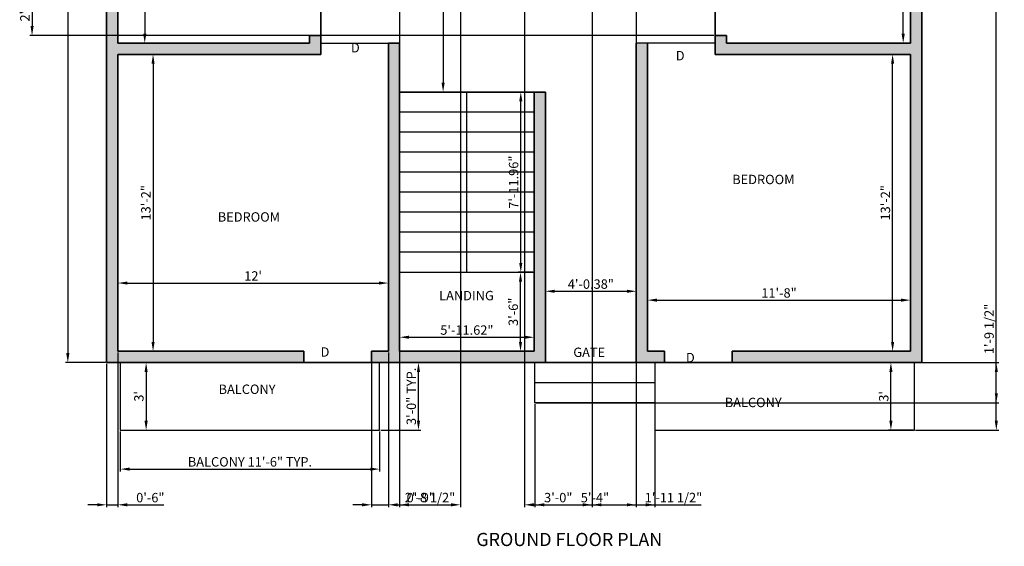
# Model space of a CAD drawing. Units: inches. Extents: x -48 to 476, y -487 to 101.
# Tile 1 of 2: x -48 to 476, y -487 to -207. Entities that reach past the tile are written whole.
import ezdxf

# ---------------------------------------------------------------- set-up
doc = ezdxf.new("R2010")
doc.units = ezdxf.units.IN
for name, color, linetype, lineweight in [('A-ANNO-DIMS', 2, 'Continuous', 18), ('A-ANNO-TEXT', 7, 'Continuous', 18), ('A-AREA-IDEN', 7, 'Continuous', 18), ('A-DOOR', 4, 'Continuous', 25), ('A-FLOR-BALC', 7, 'Continuous', 25), ('A-FLOR-STRS', 7, 'Continuous', 25), ('A-WALL', 7, 'Continuous', 35), ('A-WALL-PATT', 1, 'Continuous', 13)]:
    doc.layers.add(name, color=color, linetype=linetype, lineweight=lineweight)
doc.styles.get("Standard").update_dxf_attribs({"font": 'arial.ttf'})
doc.dimstyles.new('ISO-25', dxfattribs={"dimtxt": 5, "dimasz": 5, "dimexe": 1.25, "dimexo": 0.625, "dimtad": 1, "dimlunit": 3, "dimtxsty": 'Standard', "dimcen": 2.5, "dimadec": 0, "dimazin": 0, "dimtfac": 1, "dimtmove": 0, "dimatfit": 3, "dimfxl": 1, "dimarcsym": 0})

# ---------------------------------------------------------------- blocks, each defined once
blk = doc.blocks.new('*D9')
at = {"layer": 'A-ANNO-DIMS', "color": 0, "lineweight": -2, "transparency": 16777216}
for p, q in [((425.39, -159.13), (420.87, -159.13)), ((422.12, -214.13), (422.12, -164.13)), ((425.39, -219.13), (420.87, -219.13))]:
    blk.add_line(p, q, dxfattribs=at)
at = {"layer": 'A-ANNO-DIMS', "color": 0, "transparency": 16777216}
for points in [[(421.29, -164.13), (422.95, -164.13), (422.12, -159.13)], [(421.29, -214.13), (422.95, -214.13), (422.12, -219.13)]]:
    blk.add_solid(points, dxfattribs=at)
at = {"layer": 'Defpoints', "color": 0, "transparency": 16777216}
for p in [(422.12, -159.13), (426.01, -159.13), (426.01, -219.13)]:
    blk.add_point(p, dxfattribs=at)
at = {"layer": 'A-ANNO-DIMS', "color": 0, "transparency": 16777216, "insert": (418.95, -189.13), "char_height": 5, "attachment_point": 5, "rotation": 90}
blk.add_mtext("5'", dxfattribs=at)
blk = doc.blocks.new('*D10')
at = {"layer": 'A-ANNO-DIMS', "color": 0, "lineweight": -2, "transparency": 16777216}
for p, q in [((286.01, -382.51), (286.01, -354.68)), ((291.01, -355.93), (421.01, -355.93)), ((426.01, -382.51), (426.01, -354.68))]:
    blk.add_line(p, q, dxfattribs=at)
at = {"layer": 'A-ANNO-DIMS', "color": 0, "transparency": 16777216}
for points in [[(291.01, -355.1), (291.01, -356.77), (286.01, -355.93)], [(421.01, -355.1), (421.01, -356.77), (426.01, -355.93)]]:
    blk.add_solid(points, dxfattribs=at)
at = {"layer": 'Defpoints', "color": 0, "transparency": 16777216}
for p in [(426.01, -355.93), (286.01, -383.13), (426.01, -383.13)]:
    blk.add_point(p, dxfattribs=at)
at = {"layer": 'A-ANNO-DIMS', "color": 0, "transparency": 16777216, "insert": (356.01, -352.75), "char_height": 5, "attachment_point": 5}
blk.add_mtext('11\'-8"', dxfattribs=at)
blk = doc.blocks.new('*D11')
at = {"layer": 'A-ANNO-DIMS', "color": 0, "lineweight": -2, "transparency": 16777216}
for p, q in [((425.39, -225.13), (415.24, -225.13)), ((416.49, -378.13), (416.49, -230.13)), ((425.39, -383.13), (415.24, -383.13))]:
    blk.add_line(p, q, dxfattribs=at)
at = {"layer": 'A-ANNO-DIMS', "color": 0, "transparency": 16777216}
for points in [[(415.66, -230.13), (417.32, -230.13), (416.49, -225.13)], [(415.66, -378.13), (417.32, -378.13), (416.49, -383.13)]]:
    blk.add_solid(points, dxfattribs=at)
at = {"layer": 'Defpoints', "color": 0, "transparency": 16777216}
for p in [(416.49, -225.13), (426.01, -225.13), (426.01, -383.13)]:
    blk.add_point(p, dxfattribs=at)
at = {"layer": 'A-ANNO-DIMS', "color": 0, "transparency": 16777216, "insert": (413.31, -304.13), "char_height": 5, "attachment_point": 5, "rotation": 90}
blk.add_mtext('13\'-2"', dxfattribs=at)
blk = doc.blocks.new('*D12')
at = {"layer": 'A-ANNO-DIMS', "color": 0, "lineweight": -2, "transparency": 16777216}
for p, q in [((431.39, -389.13), (414.33, -389.13)), ((415.58, -420.13), (415.58, -394.13)), ((427.51, -425.13), (414.33, -425.13))]:
    blk.add_line(p, q, dxfattribs=at)
at = {"layer": 'A-ANNO-DIMS', "color": 0, "transparency": 16777216}
for points in [[(414.75, -394.13), (416.42, -394.13), (415.58, -389.13)], [(414.75, -420.13), (416.42, -420.13), (415.58, -425.13)]]:
    blk.add_solid(points, dxfattribs=at)
at = {"layer": 'Defpoints', "color": 0, "transparency": 16777216}
for p in [(415.58, -389.13), (432.01, -389.13), (428.14, -425.13)]:
    blk.add_point(p, dxfattribs=at)
at = {"layer": 'A-ANNO-DIMS', "color": 0, "transparency": 16777216, "insert": (412.4, -407.13), "char_height": 5, "attachment_point": 5, "rotation": 90}
blk.add_mtext("3'", dxfattribs=at)
blk = doc.blocks.new('*D13')
at = {"layer": 'A-ANNO-DIMS', "color": 0, "lineweight": -2, "transparency": 16777216}
for p, q in [((231.63, -350.58), (231.63, -349.96)), ((236.63, -351.21), (275.01, -351.21)), ((280.01, -350.58), (280.01, -349.96))]:
    blk.add_line(p, q, dxfattribs=at)
at = {"layer": 'A-ANNO-DIMS', "color": 0, "transparency": 16777216}
for points in [[(236.63, -350.37), (236.63, -352.04), (231.63, -351.21)], [(275.01, -350.37), (275.01, -352.04), (280.01, -351.21)]]:
    blk.add_solid(points, dxfattribs=at)
at = {"layer": 'Defpoints', "color": 0, "transparency": 16777216}
for p in [(231.63, -351.21), (280.01, -351.21), (280.01, -351.21)]:
    blk.add_point(p, dxfattribs=at)
at = {"layer": 'A-ANNO-DIMS', "color": 0, "transparency": 16777216, "insert": (255.82, -348.03), "char_height": 5, "attachment_point": 5}
blk.add_mtext('4\'-0.38"', dxfattribs=at)
blk = doc.blocks.new('*D14')
at = {"layer": 'A-ANNO-DIMS', "color": 0, "lineweight": -2, "transparency": 16777216}
for p, q in [((154.01, -382.51), (154.01, -374.42)), ((159.01, -375.67), (220.63, -375.67)), ((225.63, -382.51), (225.63, -374.42))]:
    blk.add_line(p, q, dxfattribs=at)
at = {"layer": 'A-ANNO-DIMS', "color": 0, "transparency": 16777216}
for points in [[(159.01, -374.84), (159.01, -376.5), (154.01, -375.67)], [(220.63, -374.84), (220.63, -376.5), (225.63, -375.67)]]:
    blk.add_solid(points, dxfattribs=at)
at = {"layer": 'Defpoints', "color": 0, "transparency": 16777216}
for p in [(225.63, -375.67), (154.01, -383.13), (225.63, -383.13)]:
    blk.add_point(p, dxfattribs=at)
at = {"layer": 'A-ANNO-DIMS', "color": 0, "transparency": 16777216, "insert": (189.82, -372.49), "char_height": 5, "attachment_point": 5}
blk.add_mtext('5\'-11.62"', dxfattribs=at)
blk = doc.blocks.new('*D15')
at = {"layer": 'A-ANNO-DIMS', "color": 0, "lineweight": -2, "transparency": 16777216}
for p, q in [((225.01, -341.13), (217.11, -341.13)), ((218.36, -378.13), (218.36, -346.13)), ((225.01, -383.13), (217.11, -383.13))]:
    blk.add_line(p, q, dxfattribs=at)
at = {"layer": 'A-ANNO-DIMS', "color": 0, "transparency": 16777216}
for points in [[(217.53, -346.13), (219.2, -346.13), (218.36, -341.13)], [(217.53, -378.13), (219.2, -378.13), (218.36, -383.13)]]:
    blk.add_solid(points, dxfattribs=at)
at = {"layer": 'Defpoints', "color": 0, "transparency": 16777216}
for p in [(218.36, -341.13), (225.63, -341.13), (225.63, -383.13)]:
    blk.add_point(p, dxfattribs=at)
at = {"layer": 'A-ANNO-DIMS', "color": 0, "transparency": 16777216, "insert": (215.18, -362.13), "char_height": 5, "attachment_point": 5, "rotation": 90}
blk.add_mtext('3\'-6"', dxfattribs=at)
blk = doc.blocks.new('*D16')
at = {"layer": 'A-ANNO-DIMS', "color": 0, "lineweight": -2, "transparency": 16777216}
for p, q in [((225.01, -245.18), (217.26, -245.18)), ((218.51, -336.13), (218.51, -250.18)), ((225.01, -341.13), (217.26, -341.13))]:
    blk.add_line(p, q, dxfattribs=at)
at = {"layer": 'A-ANNO-DIMS', "color": 0, "transparency": 16777216}
for points in [[(217.68, -250.18), (219.34, -250.18), (218.51, -245.18)], [(217.68, -336.13), (219.34, -336.13), (218.51, -341.13)]]:
    blk.add_solid(points, dxfattribs=at)
at = {"layer": 'Defpoints', "color": 0, "transparency": 16777216}
for p in [(218.51, -245.18), (225.63, -245.18), (225.63, -341.13)]:
    blk.add_point(p, dxfattribs=at)
at = {"layer": 'A-ANNO-DIMS', "color": 0, "transparency": 16777216, "insert": (215.33, -293.15), "char_height": 5, "attachment_point": 5, "rotation": 90}
blk.add_mtext('7\'-11.96"', dxfattribs=at)
blk = doc.blocks.new('*D17')
at = {"layer": 'A-ANNO-DIMS', "color": 0, "lineweight": -2, "transparency": 16777216}
for p, q in [((5.92, -389.13), (20.28, -389.13)), ((19.03, -394.13), (19.03, -420.13)), ((5.92, -425.13), (20.28, -425.13))]:
    blk.add_line(p, q, dxfattribs=at)
at = {"layer": 'A-ANNO-DIMS', "color": 0, "transparency": 16777216}
for points in [[(18.2, -394.13), (19.87, -394.13), (19.03, -389.13)], [(18.2, -420.13), (19.87, -420.13), (19.03, -425.13)]]:
    blk.add_solid(points, dxfattribs=at)
at = {"layer": 'Defpoints', "color": 0, "transparency": 16777216}
for p in [(5.3, -389.13), (5.3, -425.13), (19.03, -425.13)]:
    blk.add_point(p, dxfattribs=at)
at = {"layer": 'A-ANNO-DIMS', "color": 0, "transparency": 16777216, "insert": (15.85, -407.13), "char_height": 5, "attachment_point": 5, "rotation": 90}
blk.add_mtext("3'", dxfattribs=at)
blk = doc.blocks.new('*D18')
at = {"layer": 'A-ANNO-DIMS', "color": 0, "lineweight": -2, "transparency": 16777216}
for p, q in [((4.01, -382.51), (4.01, -345.58)), ((148.01, -382.51), (148.01, -345.58)), ((9.01, -346.83), (143.01, -346.83))]:
    blk.add_line(p, q, dxfattribs=at)
at = {"layer": 'A-ANNO-DIMS', "color": 0, "transparency": 16777216}
for points in [[(9.01, -346), (9.01, -347.67), (4.01, -346.83)], [(143.01, -346), (143.01, -347.67), (148.01, -346.83)]]:
    blk.add_solid(points, dxfattribs=at)
at = {"layer": 'Defpoints', "color": 0, "transparency": 16777216}
for p in [(148.01, -346.83), (4.01, -383.13), (148.01, -383.13)]:
    blk.add_point(p, dxfattribs=at)
at = {"layer": 'A-ANNO-DIMS', "color": 0, "transparency": 16777216, "insert": (76.01, -343.7), "char_height": 5, "attachment_point": 5}
blk.add_mtext("12'", dxfattribs=at)
blk = doc.blocks.new('*D19')
at = {"layer": 'A-ANNO-DIMS', "color": 0, "lineweight": -2, "transparency": 16777216}
for p, q in [((4.64, -225.13), (23.98, -225.13)), ((22.73, -230.13), (22.73, -378.13)), ((4.64, -383.13), (23.98, -383.13))]:
    blk.add_line(p, q, dxfattribs=at)
at = {"layer": 'A-ANNO-DIMS', "color": 0, "transparency": 16777216}
for points in [[(21.9, -230.13), (23.56, -230.13), (22.73, -225.13)], [(21.9, -378.13), (23.56, -378.13), (22.73, -383.13)]]:
    blk.add_solid(points, dxfattribs=at)
at = {"layer": 'Defpoints', "color": 0, "transparency": 16777216}
for p in [(4.01, -225.13), (4.01, -383.13), (22.73, -383.13)]:
    blk.add_point(p, dxfattribs=at)
at = {"layer": 'A-ANNO-DIMS', "color": 0, "transparency": 16777216, "insert": (19.55, -304.13), "char_height": 5, "attachment_point": 5, "rotation": 90}
blk.add_mtext('13\'-2"', dxfattribs=at)
blk = doc.blocks.new('*D21')
at = {"layer": 'A-ANNO-DIMS', "color": 0, "lineweight": -2, "transparency": 16777216}
for p, q in [((4.64, -159.13), (19.56, -159.13)), ((18.31, -164.13), (18.31, -214.13)), ((4.64, -219.13), (19.56, -219.13))]:
    blk.add_line(p, q, dxfattribs=at)
at = {"layer": 'A-ANNO-DIMS', "color": 0, "transparency": 16777216}
for points in [[(17.48, -164.13), (19.15, -164.13), (18.31, -159.13)], [(17.48, -214.13), (19.15, -214.13), (18.31, -219.13)]]:
    blk.add_solid(points, dxfattribs=at)
at = {"layer": 'Defpoints', "color": 0, "transparency": 16777216}
for p in [(4.01, -159.13), (4.01, -219.13), (18.31, -219.13)]:
    blk.add_point(p, dxfattribs=at)
at = {"layer": 'A-ANNO-DIMS', "color": 0, "transparency": 16777216, "insert": (15.14, -189.13), "char_height": 5, "attachment_point": 5, "rotation": 90}
blk.add_mtext("5'", dxfattribs=at)
blk = doc.blocks.new('*D22')
at = {"layer": 'A-ANNO-DIMS', "color": 0, "lineweight": -2, "transparency": 16777216}
for p, q in [((154.64, -93.13), (178.42, -93.13)), ((177.17, -98.13), (177.17, -240.18)), ((154.64, -245.18), (178.42, -245.18))]:
    blk.add_line(p, q, dxfattribs=at)
at = {"layer": 'A-ANNO-DIMS', "color": 0, "transparency": 16777216}
for points in [[(176.34, -98.13), (178, -98.13), (177.17, -93.13)], [(176.34, -240.18), (178, -240.18), (177.17, -245.18)]]:
    blk.add_solid(points, dxfattribs=at)
at = {"layer": 'Defpoints', "color": 0, "transparency": 16777216}
for p in [(154.01, -93.13), (154.01, -245.18), (177.17, -245.18)]:
    blk.add_point(p, dxfattribs=at)
at = {"layer": 'A-ANNO-DIMS', "color": 0, "transparency": 16777216, "insert": (173.99, -169.15), "char_height": 5, "attachment_point": 5, "rotation": 90}
blk.add_mtext('12\'-8.04"', dxfattribs=at)
blk = doc.blocks.new('*D26')
at = {"layer": 'A-ANNO-DIMS', "color": 0, "lineweight": -2, "transparency": 16777216}
for p, q in [((-2.61, 14.87), (-23.89, 14.87)), ((-22.64, 9.87), (-22.64, -384.13)), ((-2.61, -389.13), (-23.89, -389.13))]:
    blk.add_line(p, q, dxfattribs=at)
at = {"layer": 'A-ANNO-DIMS', "color": 0, "transparency": 16777216}
for points in [[(-23.48, 9.87), (-21.81, 9.87), (-22.64, 14.87)], [(-23.48, -384.13), (-21.81, -384.13), (-22.64, -389.13)]]:
    blk.add_solid(points, dxfattribs=at)
at = {"layer": 'Defpoints', "color": 0, "transparency": 16777216}
for p in [(-1.99, 14.87), (-22.64, -389.13), (-1.99, -389.13)]:
    blk.add_point(p, dxfattribs=at)
at = {"layer": 'A-ANNO-DIMS', "color": 0, "transparency": 16777216, "insert": (-25.82, -187.13), "char_height": 5, "attachment_point": 5, "rotation": 90}
blk.add_mtext('33\'-8"', dxfattribs=at)
blk = doc.blocks.new('BALCONY-EDGE-REAR')
for p, q in [((0, 0), (0, -36)), ((138.05, -36), (138.05, 0)), ((0, -36), (138.05, -36))]:
    blk.add_line(p, q)
blk = doc.blocks.new('DOOR-36-CLOSED')
blk.add_line((0, 0), (36, 0))
blk = doc.blocks.new('*D31')
at = {"layer": 'A-ANNO-DIMS', "color": 0, "lineweight": -2, "transparency": 16777216}
for p, q in [((5.3, -425.76), (5.3, -447.09)), ((143.34, -425.76), (143.34, -447.09)), ((10.3, -445.84), (138.34, -445.84))]:
    blk.add_line(p, q, dxfattribs=at)
at = {"layer": 'A-ANNO-DIMS', "color": 0, "transparency": 16777216}
for points in [[(10.3, -445.01), (10.3, -446.67), (5.3, -445.84)], [(138.34, -445.01), (138.34, -446.67), (143.34, -445.84)]]:
    blk.add_solid(points, dxfattribs=at)
at = {"layer": 'Defpoints', "color": 0, "transparency": 16777216}
for p in [(5.3, -425.13), (143.34, -425.13), (143.34, -445.84)]:
    blk.add_point(p, dxfattribs=at)
at = {"layer": 'A-ANNO-DIMS', "color": 0, "transparency": 16777216, "insert": (74.32, -442.63), "char_height": 5, "attachment_point": 5}
blk.add_mtext('BALCONY 11\'-6" TYP.', dxfattribs=at)
blk = doc.blocks.new('*D32')
at = {"layer": 'A-ANNO-DIMS', "color": 0, "lineweight": -2, "transparency": 16777216}
for p, q in [((143.97, -389.13), (165.3, -389.13)), ((164.05, -420.13), (164.05, -394.13)), ((143.97, -425.13), (165.3, -425.13))]:
    blk.add_line(p, q, dxfattribs=at)
at = {"layer": 'A-ANNO-DIMS', "color": 0, "transparency": 16777216}
for points in [[(163.22, -394.13), (164.88, -394.13), (164.05, -389.13)], [(163.22, -420.13), (164.88, -420.13), (164.05, -425.13)]]:
    blk.add_solid(points, dxfattribs=at)
at = {"layer": 'Defpoints', "color": 0, "transparency": 16777216}
for p in [(143.34, -389.13), (164.05, -389.13), (143.34, -425.13)]:
    blk.add_point(p, dxfattribs=at)
at = {"layer": 'A-ANNO-DIMS', "color": 0, "transparency": 16777216, "insert": (160.87, -407.13), "char_height": 5, "attachment_point": 5, "rotation": 90}
blk.add_mtext('3\'-0" TYP.', dxfattribs=at)
blk = doc.blocks.new('*D33')
at = {"layer": 'A-ANNO-DIMS', "color": 0, "lineweight": -2, "transparency": 16777216}
for p, q in [((428.77, 50.87), (472.96, 50.87)), ((471.71, -420.13), (471.71, 45.87)), ((428.76, -425.13), (472.96, -425.13))]:
    blk.add_line(p, q, dxfattribs=at)
at = {"layer": 'A-ANNO-DIMS', "color": 0, "transparency": 16777216}
for points in [[(470.88, 45.87), (472.54, 45.87), (471.71, 50.87)], [(470.88, -420.13), (472.54, -420.13), (471.71, -425.13)]]:
    blk.add_solid(points, dxfattribs=at)
at = {"layer": 'Defpoints', "color": 0, "transparency": 16777216}
for p in [(428.14, 50.87), (471.71, 50.87), (428.14, -425.13)]:
    blk.add_point(p, dxfattribs=at)
at = {"layer": 'A-ANNO-DIMS', "color": 0, "transparency": 16777216, "insert": (468.53, -187.13), "char_height": 5, "attachment_point": 5, "rotation": 90}
blk.add_mtext('39\'-8"', dxfattribs=at)
blk = doc.blocks.new('*D36')
at = {"layer": 'A-ANNO-DIMS', "color": 0, "lineweight": -2, "transparency": 16777216}
for p, q in [((154.01, -87.76), (154.01, -466.08)), ((186.37, -87.76), (186.37, -466.08)), ((159.01, -464.83), (181.37, -464.83))]:
    blk.add_line(p, q, dxfattribs=at)
at = {"layer": 'A-ANNO-DIMS', "color": 0, "transparency": 16777216}
for points in [[(159.01, -464), (159.01, -465.67), (154.01, -464.83)], [(181.37, -464), (181.37, -465.67), (186.37, -464.83)]]:
    blk.add_solid(points, dxfattribs=at)
at = {"layer": 'Defpoints', "color": 0, "transparency": 16777216}
for p in [(154.01, -87.13), (186.37, -87.13), (186.37, -464.83)]:
    blk.add_point(p, dxfattribs=at)
at = {"layer": 'A-ANNO-DIMS', "color": 0, "transparency": 16777216, "insert": (170.19, -461.62), "char_height": 5, "attachment_point": 5}
blk.add_mtext('2\'-8 1/2"', dxfattribs=at)
blk = doc.blocks.new('*D37')
at = {"layer": 'A-ANNO-DIMS', "color": 0, "lineweight": -2, "transparency": 16777216}
for p, q in [((256.47, -87.76), (256.47, -466.08)), ((280.01, -87.76), (280.01, -466.08)), ((261.47, -464.83), (275.01, -464.83)), ((280.01, -464.83), (314.62, -464.83))]:
    blk.add_line(p, q, dxfattribs=at)
at = {"layer": 'A-ANNO-DIMS', "color": 0, "transparency": 16777216}
for points in [[(261.47, -464), (261.47, -465.67), (256.47, -464.83)], [(275.01, -464), (275.01, -465.67), (280.01, -464.83)]]:
    blk.add_solid(points, dxfattribs=at)
at = {"layer": 'Defpoints', "color": 0, "transparency": 16777216}
for p in [(256.47, -87.13), (280.01, -87.13), (280.01, -464.83)]:
    blk.add_point(p, dxfattribs=at)
at = {"layer": 'A-ANNO-DIMS', "color": 0, "transparency": 16777216, "insert": (299.81, -461.62), "char_height": 5, "attachment_point": 5}
blk.add_mtext('1\'-11 1/2"', dxfattribs=at)
blk = doc.blocks.new('*D39')
at = {"layer": 'A-ANNO-DIMS', "color": 0, "lineweight": -2, "transparency": 16777216}
for p, q in [((220.47, -93.76), (220.47, -466.08)), ((256.47, -93.76), (256.47, -466.08)), ((225.47, -464.83), (251.47, -464.83))]:
    blk.add_line(p, q, dxfattribs=at)
at = {"layer": 'A-ANNO-DIMS', "color": 0, "transparency": 16777216}
for points in [[(225.47, -464), (225.47, -465.67), (220.47, -464.83)], [(251.47, -464), (251.47, -465.67), (256.47, -464.83)]]:
    blk.add_solid(points, dxfattribs=at)
at = {"layer": 'Defpoints', "color": 0, "transparency": 16777216}
for p in [(220.47, -93.13), (256.47, -93.13), (256.47, -464.83)]:
    blk.add_point(p, dxfattribs=at)
at = {"layer": 'A-ANNO-DIMS', "color": 0, "transparency": 16777216, "insert": (238.47, -461.65), "char_height": 5, "attachment_point": 5}
blk.add_mtext('3\'-0"', dxfattribs=at)
blk = doc.blocks.new('*D40')
at = {"layer": 'A-ANNO-DIMS', "color": 0, "lineweight": -2, "transparency": 16777216}
for p, q in [((4.01, -383.76), (4.01, -466.08)), ((-1.99, -389.76), (-1.99, -466.08)), ((-6.99, -464.83), (-11.99, -464.83)), ((-1.99, -464.83), (4.01, -464.83)), ((9.01, -464.83), (28.55, -464.83))]:
    blk.add_line(p, q, dxfattribs=at)
at = {"layer": 'A-ANNO-DIMS', "color": 0, "transparency": 16777216}
for points in [[(-6.99, -464), (-6.99, -465.67), (-1.99, -464.83)], [(9.01, -464), (9.01, -465.67), (4.01, -464.83)]]:
    blk.add_solid(points, dxfattribs=at)
at = {"layer": 'Defpoints', "color": 0, "transparency": 16777216}
for p in [(4.01, -383.13), (-1.99, -389.13), (4.01, -464.83)]:
    blk.add_point(p, dxfattribs=at)
at = {"layer": 'A-ANNO-DIMS', "color": 0, "transparency": 16777216, "insert": (21.28, -461.66), "char_height": 5, "attachment_point": 5}
blk.add_mtext('0\'-6"', dxfattribs=at)
blk = doc.blocks.new('*D42')
at = {"layer": 'A-ANNO-DIMS', "color": 0, "lineweight": -2, "transparency": 16777216}
for p, q in [((321.39, -185.13), (-42.94, -185.13)), ((-41.69, -190.13), (-41.69, -210.13)), ((321.39, -215.13), (-42.94, -215.13))]:
    blk.add_line(p, q, dxfattribs=at)
at = {"layer": 'A-ANNO-DIMS', "color": 0, "transparency": 16777216}
for points in [[(-42.52, -190.13), (-40.86, -190.13), (-41.69, -185.13)], [(-42.52, -210.13), (-40.86, -210.13), (-41.69, -215.13)]]:
    blk.add_solid(points, dxfattribs=at)
at = {"layer": 'Defpoints', "color": 0, "transparency": 16777216}
for p in [(322.01, -185.13), (-41.69, -215.13), (322.01, -215.13)]:
    blk.add_point(p, dxfattribs=at)
at = {"layer": 'A-ANNO-DIMS', "color": 0, "transparency": 16777216, "insert": (-44.87, -200.13), "char_height": 5, "attachment_point": 5, "rotation": 90}
blk.add_mtext('2\'-6"', dxfattribs=at)
blk = doc.blocks.new('*D43')
at = {"layer": 'A-ANNO-DIMS', "color": 0, "lineweight": -2, "transparency": 16777216}
for p, q in [((226.04, -411.13), (226.04, -466.08)), ((289.97, -411.13), (289.97, -466.08)), ((231.04, -464.83), (284.97, -464.83))]:
    blk.add_line(p, q, dxfattribs=at)
at = {"layer": 'A-ANNO-DIMS', "color": 0, "transparency": 16777216}
for points in [[(231.04, -464), (231.04, -465.67), (226.04, -464.83)], [(284.97, -464), (284.97, -465.67), (289.97, -464.83)]]:
    blk.add_solid(points, dxfattribs=at)
at = {"layer": 'Defpoints', "color": 0, "transparency": 16777216}
for p in [(226.04, -410.5), (289.97, -410.5), (289.97, -464.83)]:
    blk.add_point(p, dxfattribs=at)
at = {"layer": 'A-ANNO-DIMS', "color": 0, "transparency": 16777216, "insert": (258, -461.67), "char_height": 5, "attachment_point": 5}
blk.add_mtext('5\'-4"', dxfattribs=at)
blk = doc.blocks.new('*D44')
at = {"layer": 'A-ANNO-DIMS', "color": 0, "lineweight": -2, "transparency": 16777216}
for p, q in [((471.71, -389.13), (471.71, -358.41)), ((226.66, -389.13), (472.96, -389.13)), ((471.71, -405.5), (471.71, -394.13)), ((226.66, -410.5), (472.96, -410.5))]:
    blk.add_line(p, q, dxfattribs=at)
at = {"layer": 'A-ANNO-DIMS', "color": 0, "transparency": 16777216}
for points in [[(470.88, -394.13), (472.54, -394.13), (471.71, -389.13)], [(470.88, -405.5), (472.54, -405.5), (471.71, -410.5)]]:
    blk.add_solid(points, dxfattribs=at)
at = {"layer": 'Defpoints', "color": 0, "transparency": 16777216}
for p in [(226.04, -389.13), (471.71, -389.13), (226.04, -410.5)]:
    blk.add_point(p, dxfattribs=at)
at = {"layer": 'A-ANNO-DIMS', "color": 0, "transparency": 16777216, "insert": (468.5, -371.27), "char_height": 5, "attachment_point": 5, "rotation": 90}
blk.add_mtext('1\'-9 1/2"', dxfattribs=at)
blk = doc.blocks.new('*D45')
at = {"layer": 'A-ANNO-DIMS', "color": 0, "lineweight": -2, "transparency": 16777216}
for p, q in [((139.01, -383.76), (139.01, -466.08)), ((148.01, -383.76), (148.01, -466.08)), ((134.01, -464.83), (129.01, -464.83)), ((139.01, -464.83), (148.01, -464.83)), ((153.01, -464.83), (172.55, -464.83))]:
    blk.add_line(p, q, dxfattribs=at)
at = {"layer": 'A-ANNO-DIMS', "color": 0, "transparency": 16777216}
for points in [[(134.01, -464), (134.01, -465.67), (139.01, -464.83)], [(153.01, -464), (153.01, -465.67), (148.01, -464.83)]]:
    blk.add_solid(points, dxfattribs=at)
at = {"layer": 'Defpoints', "color": 0, "transparency": 16777216}
for p in [(139.01, -383.13), (148.01, -383.13), (148.01, -464.83)]:
    blk.add_point(p, dxfattribs=at)
at = {"layer": 'A-ANNO-DIMS', "color": 0, "transparency": 16777216, "insert": (165.28, -461.66), "char_height": 5, "attachment_point": 5}
blk.add_mtext('0\'-9"', dxfattribs=at)

msp = doc.modelspace()

# ---------------------------------------------------------------- hatches: boundary and pattern name
at = {"layer": 'A-WALL-PATT'}
h = msp.add_hatch(color=256, dxfattribs=at)
h.dxf.hatch_style = 1
h.paths.add_polyline_path([(103.011, 14.867), (-1.989, 14.867), (-1.989, -389.133), (103.011, -389.133), (103.011, -383.133), (4.011, -383.133), (4.011, -225.133), (112.011, -225.133), (112.011, -215.133), (106.011, -215.133), (106.011, -219.133), (4.011, -219.133), (4.011, -159.133), (106.011, -159.133), (106.011, -185.133), (112.011, -185.133), (112.011, -159.133), (112.011, -153.133), (4.011, -153.133), (4.011, 8.867), (103.011, 8.867)])
h.paths.add_polyline_path([(295.011, 14.867), (139.011, 14.867), (139.011, 8.867), (148.011, 8.867), (148.011, -159.133), (154.011, -159.133), (154.011, -93.133), (220.474, -93.133), (220.474, -87.133), (154.011, -87.133), (154.011, 8.867), (280.011, 8.867), (280.011, -87.133), (256.474, -87.133), (256.474, -93.133), (280.011, -93.133), (280.011, -159.133), (286.011, -159.133), (286.011, 8.867), (295.011, 8.867)])
h.paths.add_polyline_path([(432.011, 14.867), (331.011, 14.867), (331.011, 8.867), (426.011, 8.867), (426.011, -153.133), (322.011, -153.133), (322.011, -159.133), (322.011, -185.133), (328.011, -185.133), (328.011, -159.133), (426.011, -159.133), (426.011, -219.133), (328.011, -219.133), (328.011, -215.133), (322.011, -215.133), (322.011, -225.133), (426.011, -225.133), (426.011, -383.133), (331.011, -383.133), (331.011, -389.133), (432.011, -389.133)])
h.paths.add_polyline_path([(295.011, -383.133), (286.011, -383.133), (286.011, -219.133), (280.011, -219.133), (280.011, -389.133), (289.971, -389.133), (295.011, -389.133)])
h.paths.add_polyline_path([(231.632, -245.175), (225.632, -245.175), (225.632, -383.133), (154.011, -383.133), (154.011, -219.133), (148.011, -219.133), (148.011, -383.133), (139.011, -383.133), (139.011, -389.133), (231.632, -389.133)])

# ---------------------------------------------------------------- linework, layer by layer
at = {"layer": 'A-DOOR'}
msp.add_line((322.011, -219.133), (280.011, -219.133), dxfattribs=at)
at = {"layer": 'A-FLOR-STRS'}
for p, q in [((225.632, -245.175), (154.011, -245.175)), ((189.821, -341.133), (189.821, -245.175)), ((225.632, -255.837), (154.011, -255.837)), ((225.632, -266.499), (154.011, -266.499)), ((225.632, -277.161), (154.011, -277.161)), ((225.632, -287.823), (154.011, -287.823)), ((225.632, -298.485), (154.011, -298.485)), ((225.632, -309.147), (154.011, -309.147)), ((225.632, -319.809), (154.011, -319.809)), ((225.632, -330.471), (154.011, -330.471)), ((225.632, -341.133), (154.011, -341.133)), ((226.036, -399.818), (289.971, -399.818))]:
    msp.add_line(p, q, dxfattribs=at)
msp.add_lwpolyline([(226.036, -389.133), (289.971, -389.133), (289.971, -410.503), (226.036, -410.503)], close=True, dxfattribs=at)
at = {"layer": 'A-WALL'}
for p, q in [((-1.989, -389.133), (-1.989, 14.867)), ((432.011, 14.867), (432.011, -389.133)), ((4.011, -219.133), (4.011, -159.133)), ((112.011, -159.133), (112.011, -225.133)), ((322.011, -159.133), (322.011, -225.133)), ((426.011, -159.133), (426.011, -219.133)), ((4.011, -219.133), (106.011, -219.133)), ((106.011, -215.133), (112.011, -215.133)), ((106.011, -215.133), (106.011, -219.133)), ((148.011, -383.133), (148.011, -219.133)), ((148.011, -219.133), (154.011, -219.133)), ((154.011, -383.133), (154.011, -219.133)), ((280.011, -389.133), (280.011, -219.133)), ((286.011, -383.133), (286.011, -219.133)), ((328.011, -215.133), (322.011, -215.133)), ((328.011, -215.133), (328.011, -219.133)), ((328.011, -219.133), (426.011, -219.133)), ((4.011, -383.133), (4.011, -225.133)), ((4.011, -225.133), (112.011, -225.133)), ((322.011, -225.133), (426.011, -225.133)), ((426.011, -225.133), (426.011, -383.133)), ((231.632, -245.175), (154.011, -245.175)), ((225.632, -383.133), (225.632, -245.175)), ((231.632, -389.133), (231.632, -245.175)), ((103.011, -383.133), (4.011, -383.133)), ((103.011, -383.133), (103.011, -389.133)), ((139.011, -383.133), (139.011, -389.133)), ((148.011, -383.133), (139.011, -383.133)), ((225.632, -383.133), (154.011, -383.133)), ((295.011, -383.133), (286.011, -383.133)), ((295.011, -383.133), (295.011, -389.133)), ((426.011, -383.133), (331.011, -383.133)), ((331.011, -383.133), (331.011, -389.133)), ((432.011, -389.133), (-1.989, -389.133))]:
    msp.add_line(p, q, dxfattribs=at)

# ---------------------------------------------------------------- block references
at = {"layer": 'A-DOOR'}
msp.add_blockref('DOOR-36-CLOSED', (112.011, -219.133), dxfattribs=at)
at = {"layer": 'A-FLOR-BALC'}
msp.add_blockref('BALCONY-EDGE-REAR', (5.297, -389.133), dxfattribs=at)
at = {"layer": 'A-FLOR-BALC', "xscale": 1.00088295234175}
msp.add_blockref('BALCONY-EDGE-REAR', (289.971, -389.133), dxfattribs=at)

# ---------------------------------------------------------------- texts
at = {"layer": 'A-ANNO-TEXT', "attachment_point": 1}
for s, width, insert, char_height in [('D', 15.0589, (128.083, -219.133), 5), ('D', 10.27647, (301.051, -223.336), 5), ('D', 19.33264, (111.937, -381.021), 5), ('GATE', 29.70284, (246.486, -381.187), 5), ('D', 10.14505, (306.443, -383.99), 5), ('GROUND FLOOR PLAN', 282.68369, (194.825, -479.786), 7)]:
    msp.add_mtext_dynamic_manual_height_columns(s, width=width, gutter_width=12.5, heights=[0], dxfattribs=dict(at, insert=insert, char_height=char_height))
at = {"layer": 'A-AREA-IDEN', "char_height": 5, "attachment_point": 1}
for s, width, insert in [('BEDROOM', 52.60864, (331.101, -289.213)), ('BEDROOM', 94.87425, (57.192, -309.149)), ('LANDING', 50.15236, (175.057, -351.013)), ('BALCONY', 70.04029, (57.633, -400.838)), ('BALCONY', 79.12106, (327.129, -407.871))]:
    msp.add_mtext_dynamic_manual_height_columns(s, width=width, gutter_width=12.5, heights=[0], dxfattribs=dict(at, insert=insert))

# ---------------------------------------------------------------- dimensions: what is measured, and where the dimension line sits
at = {"layer": 'A-ANNO-DIMS'}
for base, p1, p2, override, picture, middle in [((471.711, 50.867), (428.139, -425.133), (428.141, 50.867), {"dimdec": 1, "dimlfac": 1, "dimrnd": 0, "dimzin": 1, "dimdsep": 46, "dimlunit": 4, "dimfrac": 2}, '*D33', (468.531, -187.133)), ((-22.642, -389.133), (-1.989, 14.867), (-1.989, -389.133), {"dimclrd": 0, "dimclre": 0, "dimclrt": 0}, '*D26', (-25.822, -187.133)), ((177.169, -245.175), (154.011, -93.133), (154.011, -245.175), {"dimclrd": 0, "dimclre": 0, "dimclrt": 0}, '*D22', (173.991, -169.154)), ((18.312, -219.133), (4.011, -159.133), (4.011, -219.133), {"dimclrd": 0, "dimclre": 0, "dimclrt": 0}, '*D21', (15.145, -189.133)), ((422.12, -159.133), (426.011, -219.133), (426.011, -159.133), {"dimclrd": 0, "dimclre": 0, "dimclrt": 0}, '*D9', (418.952, -189.133)), ((-41.689, -215.133), (322.011, -185.133), (322.011, -215.133), {"dimdec": 1, "dimlfac": 1, "dimrnd": 0, "dimzin": 1, "dimdsep": 46, "dimlunit": 4, "dimfrac": 2}, '*D42', (-44.867, -200.133)), ((22.729, -383.133), (4.011, -225.133), (4.011, -383.133), {"dimclrd": 0, "dimclre": 0, "dimclrt": 0}, '*D19', (19.55, -304.133)), ((416.489, -225.133), (426.011, -383.133), (426.011, -225.133), {"dimclrd": 0, "dimclre": 0, "dimclrt": 0}, '*D11', (413.31, -304.133)), ((218.51, -245.175), (225.632, -341.133), (225.632, -245.175), {"dimclrd": 0, "dimclre": 0, "dimclrt": 0}, '*D16', (215.332, -293.154)), ((218.363, -341.133), (225.632, -383.133), (225.632, -341.133), {"dimclrd": 0, "dimclre": 0, "dimclrt": 0}, '*D15', (215.183, -362.133)), ((471.711, -389.133), (226.036, -410.503), (226.036, -389.133), {"dimdec": 1, "dimlfac": 1, "dimrnd": 0, "dimzin": 1, "dimdsep": 46, "dimlunit": 4, "dimfrac": 2}, '*D44', (468.5, -371.272)), ((19.035, -425.133), (5.297, -389.133), (5.297, -425.133), {"dimclrd": 0, "dimclre": 0, "dimclrt": 0}, '*D17', (15.855, -407.133)), ((415.582, -389.133), (428.139, -425.133), (432.011, -389.133), {"dimclrd": 0, "dimclre": 0, "dimclrt": 0}, '*D12', (412.402, -407.133))]:
    dim = msp.add_linear_dim(base=base, p1=p1, p2=p2, angle=90, dimstyle='ISO-25', override=override, dxfattribs=at)
    dim.commit()
    dim.dimension.update_dxf_attribs({"geometry": picture, "text_midpoint": middle})
for base, p1, p2, override, picture, middle in [((186.373, -464.833), (154.011, -87.133), (186.373, -87.133), {"dimdec": 1, "dimlfac": 1, "dimrnd": 0, "dimzin": 1, "dimdsep": 46, "dimlunit": 4, "dimfrac": 2}, '*D36', (170.192, -461.623)), ((280.011, -464.833), (256.474, -87.133), (280.011, -87.133), {"dimdec": 1, "dimlfac": 1, "dimrnd": 0, "dimzin": 1, "dimdsep": 46, "dimlunit": 4, "dimfrac": 2}, '*D37', (299.814, -461.623)), ((256.474, -464.833), (220.474, -93.133), (256.474, -93.133), {"dimdec": 1, "dimlfac": 1, "dimrnd": 0, "dimzin": 1, "dimdsep": 46, "dimlunit": 4, "dimfrac": 2}, '*D39', (238.474, -461.653)), ((148.011, -346.833), (4.011, -383.133), (148.011, -383.133), {"dimclrd": 0, "dimclre": 0, "dimclrt": 0}, '*D18', (76.011, -343.698)), ((280.011, -351.208), (231.632, -351.208), (280.011, -351.208), {"dimclrd": 0, "dimclre": 0, "dimclrt": 0}, '*D13', (255.821, -348.028)), ((426.011, -355.933), (286.011, -383.133), (426.011, -383.133), {"dimclrd": 0, "dimclre": 0, "dimclrt": 0}, '*D10', (356.011, -352.755)), ((225.632, -375.671), (154.011, -383.133), (225.632, -383.133), {"dimclrd": 0, "dimclre": 0, "dimclrt": 0}, '*D14', (189.821, -372.493)), ((4.011, -464.833), (-1.989, -389.133), (4.011, -383.133), {"dimdec": 1, "dimlfac": 1, "dimrnd": 0, "dimzin": 1, "dimdsep": 46, "dimlunit": 4, "dimfrac": 2}, '*D40', (21.281, -461.655)), ((148.011, -464.833), (139.011, -383.133), (148.011, -383.133), {"dimdec": 1, "dimlfac": 1, "dimrnd": 0, "dimzin": 1, "dimdsep": 46, "dimlunit": 4, "dimfrac": 2}, '*D45', (165.281, -461.655)), ((289.971, -464.833), (226.036, -410.503), (289.971, -410.503), {"dimdec": 1, "dimlfac": 1, "dimrnd": 0, "dimzin": 1, "dimdsep": 46, "dimlunit": 4, "dimfrac": 2}, '*D43', (258.003, -461.665))]:
    dim = msp.add_linear_dim(base=base, p1=p1, p2=p2, dimstyle='ISO-25', override=override, dxfattribs=at)
    dim.commit()
    dim.dimension.update_dxf_attribs({"geometry": picture, "text_midpoint": middle})
dim = msp.add_linear_dim(base=(164.051, -389.133), p1=(143.344, -425.133), p2=(143.344, -389.133), angle=90, text='<> TYP.', dimstyle='ISO-25', override={"dimdec": 1, "dimlfac": 1, "dimrnd": 0, "dimzin": 1, "dimdsep": 46, "dimlunit": 4, "dimfrac": 2}, dxfattribs=at)
dim.commit()
dim.dimension.update_dxf_attribs({"geometry": '*D32', "text_midpoint": (160.871, -407.133)})
dim = msp.add_linear_dim(base=(143.344, -445.84), p1=(5.297, -425.133), p2=(143.344, -425.133), text='BALCONY <> TYP.', dimstyle='ISO-25', override={"dimdec": 1, "dimlfac": 1, "dimrnd": 0, "dimzin": 1, "dimdsep": 46, "dimlunit": 4, "dimfrac": 2}, dxfattribs=at)
dim.commit()
dim.dimension.update_dxf_attribs({"geometry": '*D31', "text_midpoint": (74.32, -442.628)})

doc.saveas('drawing.dxf')
